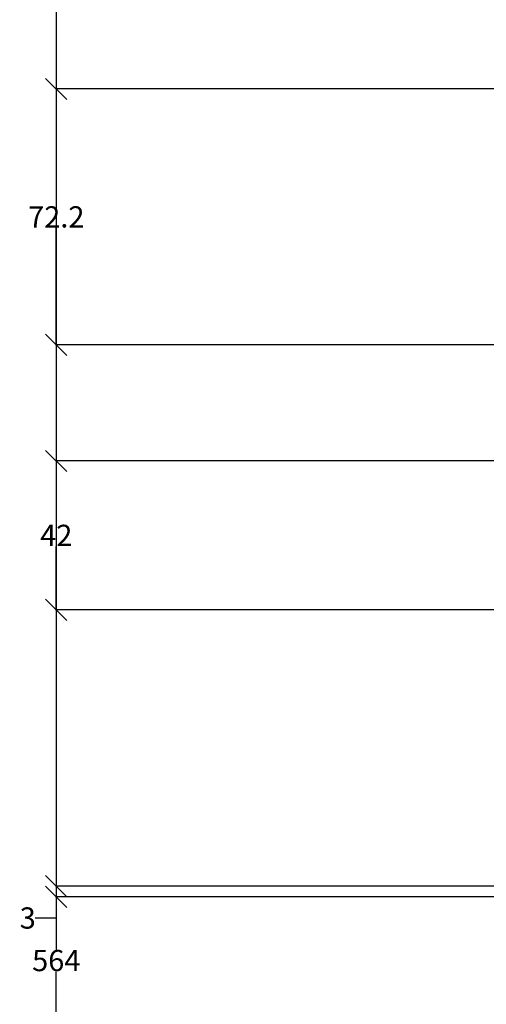
# Model space of a CAD drawing. Units: inches. Extents: x -1198 to -69, y -512 to 437.
# Tile 3 of 50: x -1198 to -1067, y 5 to 283. Entities that reach past the tile are written whole.
import ezdxf

# ---------------------------------------------------------------- set-up
doc = ezdxf.new("R2010")
doc.units = ezdxf.units.IN
doc.header["$MEASUREMENT"] = 0
doc.layers.add('A-ANNO-DIMS', color=2, linetype='Continuous', lineweight=18)
doc.styles.get("Standard").update_dxf_attribs({"font": 'arial.ttf'})
doc.dimstyles.get("Standard").update_dxf_attribs({"dimtxt": 6, "dimasz": 6, "dimexe": 0.18, "dimexo": 0.0625, "dimgap": 0.09, "dimtad": 0, "dimtih": 1, "dimtoh": 1, "dimdec": 0, "dimzin": 0, "dimdsep": 46, "dimlunit": 4, "dimtxsty": 'Standard', "dimblk": 'OBLIQUE', "dimcen": 0.09, "dimadec": 0, "dimazin": 0, "dimtfac": 1, "dimtdec": 0, "dimtofl": 0, "dimtmove": 0, "dimatfit": 3, "dimfxl": 1, "dimtolj": 1, "dimtzin": 0, "dimarcsym": 0})

# ---------------------------------------------------------------- blocks, each defined once
blk = doc.blocks.new('_Oblique')
at = {"color": 0, "linetype": 'ByBlock', "lineweight": -2}
blk.add_line((-0.5, -0.5), (0.5, 0.5), dxfattribs=at)
blk = doc.blocks.new('*D61')
at = {"layer": 'A-ANNO-DIMS', "color": 0, "lineweight": -2, "ltscale": 10, "transparency": 16777216}
for p, q in [((-1054.81, 299.23), (-1188.2, 299.23)), ((-1188.02, 299.23), (-1188.02, 20.38)), ((-1188.02, -264.77), (-1188.02, 14.07)), ((-1054.81, -264.77), (-1188.2, -264.77))]:
    blk.add_line(p, q, dxfattribs=at)
at = {"layer": 'DEFPOINTS', "color": 0, "ltscale": 10, "transparency": 16777216}
for p in [(-1054.75, 299.23), (-1188.02, -264.77), (-1054.75, -264.77)]:
    blk.add_point(p, dxfattribs=at)
at = {"layer": 'A-ANNO-DIMS', "color": 0, "lineweight": -2, "ltscale": 10, "transparency": 16777216, "xscale": 6, "yscale": 6, "zscale": 6}
for p, rotation in [((-1188.02, 299.23), 90), ((-1188.02, -264.77), 270)]:
    blk.add_blockref('_Oblique', p, dxfattribs=dict(at, rotation=rotation))
at = {"layer": 'A-ANNO-DIMS', "color": 0, "ltscale": 10, "transparency": 16777216, "insert": (-1188.02, 17.23), "char_height": 6, "attachment_point": 5}
blk.add_mtext('\\A1;564', dxfattribs=at)
blk = doc.blocks.new('*D74')
at = {"layer": 'A-ANNO-DIMS', "color": 0, "lineweight": -2, "ltscale": 10, "transparency": 16777216}
for p, q in [((-1012.81, 38.23), (-1188.2, 38.23)), ((-1188.02, 38.23), (-1188.02, 35.23)), ((-1012.81, 35.23), (-1188.2, 35.23)), ((-1188.02, 35.23), (-1188.02, 29.23)), ((-1188.02, 29.23), (-1194.02, 29.23))]:
    blk.add_line(p, q, dxfattribs=at)
at = {"layer": 'DEFPOINTS', "color": 0, "ltscale": 10, "transparency": 16777216}
for p in [(-1012.75, 38.23), (-1188.02, 35.23), (-1012.75, 35.23)]:
    blk.add_point(p, dxfattribs=at)
at = {"layer": 'A-ANNO-DIMS', "color": 0, "lineweight": -2, "ltscale": 10, "transparency": 16777216, "xscale": 6, "yscale": 6, "zscale": 6}
for p, rotation in [((-1188.02, 38.23), 90), ((-1188.02, 35.23), 270)]:
    blk.add_blockref('_Oblique', p, dxfattribs=dict(at, rotation=rotation))
at = {"layer": 'A-ANNO-DIMS', "color": 0, "ltscale": 10, "transparency": 16777216, "insert": (-1196.08, 29.23), "char_height": 6, "attachment_point": 5}
blk.add_mtext('\\A1;3', dxfattribs=at)
blk = doc.blocks.new('*D80')
at = {"layer": 'A-ANNO-DIMS', "color": 0, "lineweight": -2, "ltscale": 10, "transparency": 16777216}
for p, q in [((-1012.81, 158.23), (-1188.2, 158.23)), ((-1188.02, 158.23), (-1188.02, 140.33)), ((-1188.02, 116.23), (-1188.02, 134.13)), ((-1018.81, 116.23), (-1188.2, 116.23))]:
    blk.add_line(p, q, dxfattribs=at)
at = {"layer": 'DEFPOINTS', "color": 0, "ltscale": 10, "transparency": 16777216}
for p in [(-1188.02, 158.23), (-1012.75, 158.23), (-1018.75, 116.23)]:
    blk.add_point(p, dxfattribs=at)
at = {"layer": 'A-ANNO-DIMS', "color": 0, "lineweight": -2, "ltscale": 10, "transparency": 16777216, "xscale": 6, "yscale": 6, "zscale": 6}
for p, rotation in [((-1188.02, 158.23), 90), ((-1188.02, 116.23), 270)]:
    blk.add_blockref('_Oblique', p, dxfattribs=dict(at, rotation=rotation))
at = {"layer": 'A-ANNO-DIMS', "color": 0, "ltscale": 10, "transparency": 16777216, "insert": (-1188.02, 137.23), "char_height": 6, "attachment_point": 5}
blk.add_mtext('\\A1;42', dxfattribs=at)
blk = doc.blocks.new('*D81')
at = {"layer": 'A-ANNO-DIMS', "color": 0, "lineweight": -2, "ltscale": 10, "transparency": 16777216}
for p, q in [((-1018.81, 263.23), (-1188.2, 263.23)), ((-1188.02, 263.23), (-1188.02, 230.23)), ((-1188.02, 191.02), (-1188.02, 224.02)), ((-1018.81, 191.02), (-1188.2, 191.02))]:
    blk.add_line(p, q, dxfattribs=at)
at = {"layer": 'DEFPOINTS', "color": 0, "ltscale": 10, "transparency": 16777216}
for p in [(-1188.02, 263.23), (-1018.75, 263.23), (-1018.75, 191.02)]:
    blk.add_point(p, dxfattribs=at)
at = {"layer": 'A-ANNO-DIMS', "color": 0, "lineweight": -2, "ltscale": 10, "transparency": 16777216, "xscale": 6, "yscale": 6, "zscale": 6}
for p, rotation in [((-1188.02, 263.23), 90), ((-1188.02, 191.02), 270)]:
    blk.add_blockref('_Oblique', p, dxfattribs=dict(at, rotation=rotation))
at = {"layer": 'A-ANNO-DIMS', "color": 0, "ltscale": 10, "transparency": 16777216, "insert": (-1188.02, 227.12), "char_height": 6, "attachment_point": 5}
blk.add_mtext('\\A1;72.2', dxfattribs=at)

msp = doc.modelspace()

# ---------------------------------------------------------------- dimensions: what is measured, and where the dimension line sits
at = {"layer": 'A-ANNO-DIMS', "ltscale": 10}
for base, p1, p2, override, picture, middle in [((-1188.0248, -264.7723), (-1054.7509, 299.2277), (-1054.7509, -264.7723), {"dimdec": 0, "dimlfac": 1, "dimrnd": 0, "dimzin": 0, "dimdsep": 46, "dimlunit": 2}, '*D61', (-1188.0248, 17.2277)), ((-1188.0248, 263.2277), (-1018.7509, 191.0212), (-1018.7509, 263.2277), {"dimdec": 1, "dimlfac": 1, "dimrnd": 0, "dimzin": 0, "dimdsep": 46, "dimlunit": 2}, '*D81', (-1188.0248, 227.1244)), ((-1188.0248, 158.2277), (-1018.7509, 116.2277), (-1012.7509, 158.2277), {"dimdec": 0, "dimlfac": 1, "dimrnd": 0, "dimzin": 0, "dimdsep": 46, "dimlunit": 2}, '*D80', (-1188.0248, 137.2277)), ((-1188.0248, 35.2277), (-1012.7509, 38.2277), (-1012.7509, 35.2277), {"dimdec": 0, "dimlfac": 1, "dimrnd": 0, "dimzin": 0, "dimdsep": 46, "dimlunit": 2}, '*D74', (-1196.0793, 29.2277))]:
    dim = msp.add_linear_dim(base=base, p1=p1, p2=p2, angle=90, dimstyle='Standard', override=override, dxfattribs=at)
    dim.commit()
    dim.dimension.update_dxf_attribs({"geometry": picture, "text_midpoint": middle})

doc.saveas('drawing.dxf')
